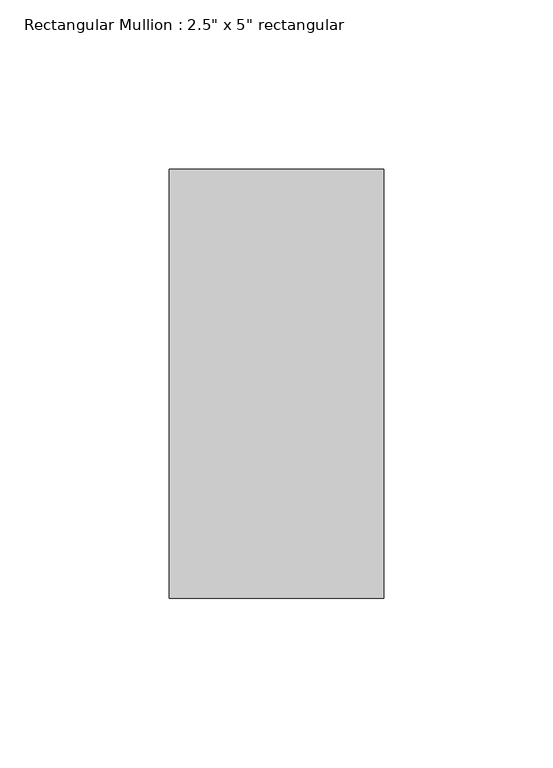
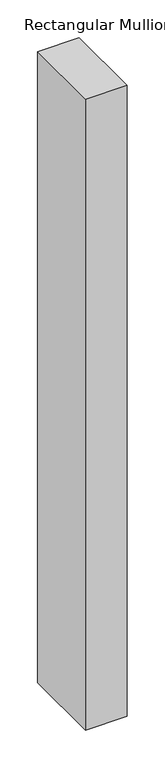
"""IFC4 building model written with IfcOpenShell, lengths in millimetres: member geometry."""

from ifc_helpers import new_model, si_unit, frame, origin, place, context, project, spatial, polyline, outline, extrude, source, transform, mapped, element, save


def member_7dabcdc2(model_context):
    return source(origin(), model_context, "Body", "SweptSolid", [
        extrude(outline(polyline([(31.75, 63.5), (31.75, -63.5), (-31.75, -63.5), (-31.75, 63.5), (31.75, 63.5)])), frame((0.0, 0.0, -1019.953622), z_axis=(0.0, 0.0, 1.0), x_axis=(1.0, 0.0, 0.0)), (0.0, 0.0, 1.0), 1019.953622),
    ])


if __name__ == "__main__":
    model = new_model("IFC4")
    model_context = context("Model", 3, world=origin())
    ifc_project = project(units=[si_unit("LENGTHUNIT", "METRE", prefix="MILLI")], contexts=[model_context])
    site = spatial("IfcSite", under=ifc_project)
    building = spatial("IfcBuilding", under=site)
    placement = place(None, origin())
    member_shape = member_7dabcdc2(model_context)
    element("IfcMember", 1, ObjectType="Rectangular Mullion : 2.5\" x 5\" rectangular", at=placement, inside=building, context=model_context, shape_type="MappedRepresentation", body=[
        mapped(member_shape, transform((0.0, 0.0, 0.0), x_axis=(1.0, 0.0, 0.0), y_axis=(0.0, 1.0, 0.0), z_axis=(0.0, 0.0, 1.0))),
    ])
    save(model, "model.ifc")

# Revit data of these elements
# Type "Rectangular Mullion : 2.5\" x 5\" rectangular"
#   built-in parameter 1007304 = 0.416667 (stored number, unit not read)
#   built-in parameter 1007301 = 0.104167 (stored number, unit not read)
#   built-in parameter 1007300 = 0.104167 (stored number, unit not read)
# Element 1 (IfcMember, "Rectangular Mullion : 2.5\" x 5\" rectangular")
#   Materials on its faces: "Aluminum"
# Materials
#   "Aluminum": class "Metal", colour RGB 247 247 247, transparency 0, Description = "Aluminum 6061", Cost = 0
